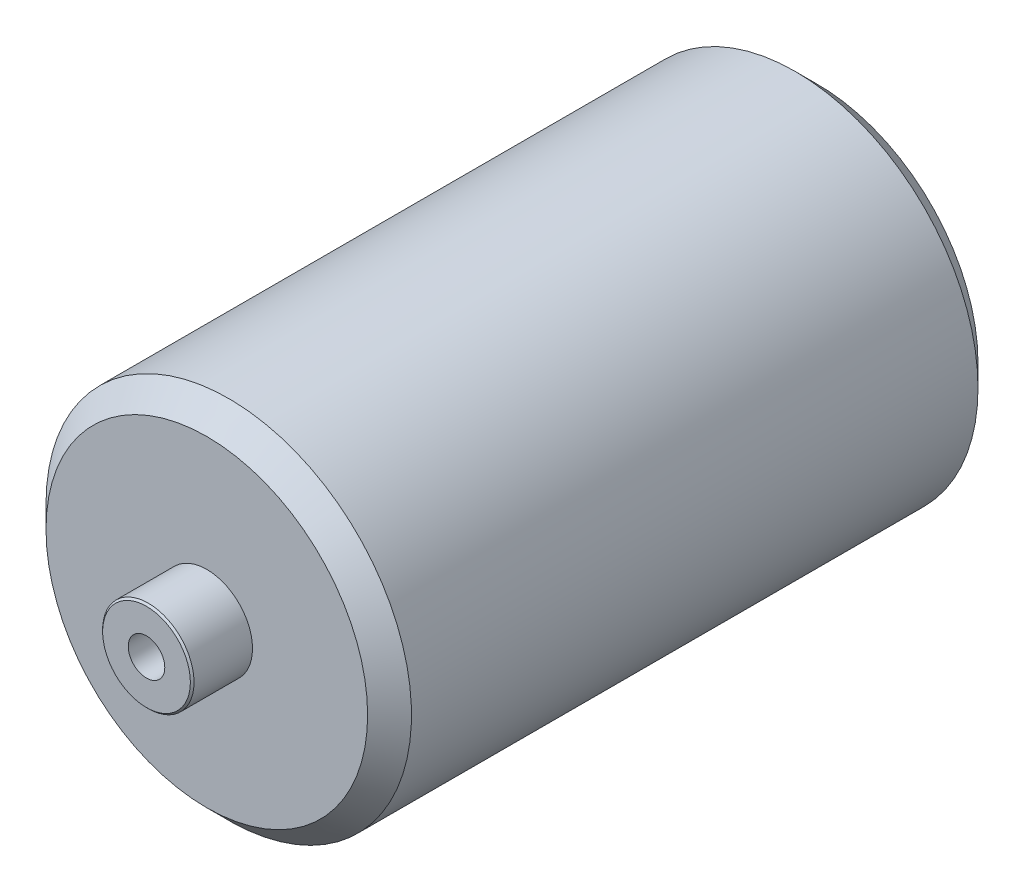
SolidWorks part; units mm, degrees
material "Plain Carbon Steel"
ref_plane "Front Plane" through (0, 0, 0) normal (0, 0, 1) x (1, 0, 0)
ref_plane "Top Plane" through (0, 0, 0) normal (0, 1, 0) x (1, 0, 0)
ref_plane "Right Plane" through (0, 0, 0) normal (1, 0, 0) x (0, 0, -1)
sketch "Body Profile Ø100" plane through (0, 0, 0) normal (0, 0, 1) x (1, 0, 0)
  circle A0 centre (0, 0) radius 50
  dimension "D1" = 100
extrude "Main Body Ø100x167" add sketch "Body Profile Ø100" along normal blind 167
sketch "Spigot 1 Profile Ø25" plane through (0, 0, 167) normal (0, 0, 1) x (1, 0, 0)
  circle A0 centre (0, 0) radius 12.5
  dimension "D1" = 25
extrude "End Spigot 1 Ø25x16.5" add sketch "Spigot 1 Profile Ø25" along normal blind 16.5
sketch "Spigot 2 Profile Ø25" plane through (0, 0, 0) normal (0, 0, -1) x (-1, 0, 0)
  circle A0 centre (0, 0) radius 12.5
  dimension "D1" = 25
extrude "End Spigot 2 Ø25x16.5" add sketch "Spigot 2 Profile Ø25" along normal blind 16.5
sketch "Spigot 2 Dowel Hole Position" plane through (0, 0, -16.5) normal (0, 0, -1) x (-1, 0, 0)
  point P0 (0, 0)
hole_wizard "Spigot 2 Dowel Hole Ø10x59" positions "3DSketch1" profile "Sketch5" hole size "Ø10.0" standard "ISO"
sketch3d "3DSketch1"
  point P0 (0, 0, -16.5)
sketch "Sketch5" plane through (0, 0, -16.5) normal (1, 0, 0) x (0, 1, 0)
  line L0 (0, 0) -> (0, 62.0043)
  line L1 (0, 62.0043) -> (5, 59)
  line L2 (5, 59) -> (5, 0)
  line L5 (5, 0) -> (0, 0)
  line L10 (0, 62.0043) -> (-5, 59) construction
  line L11 (0, -6.35) -> (0, 107.95) construction
  dimension "Hole Dia." = 10
  dimension "Hole Depth" = 59
  dimension "Drill Angle" = 118
sketch "Spigot 1 Dowel Hole Position" plane through (0, 0, 183.5) normal (0, 0, 1) x (1, 0, 0)
  point P0 (0, 0)
hole_wizard "Spigot 1 Dowel Hole Ø10x59" positions "3DSketch3" profile "Sketch9" hole size "Ø10.0" standard "ISO"
sketch3d "3DSketch3"
  point P0 (0, 0, 183.5)
sketch "Sketch9" plane through (0, 0, 183.5) normal (1, 0, 0) x (0, -1, 0)
  line L0 (0, 0) -> (0, 62.0043)
  line L1 (0, 62.0043) -> (5, 59)
  line L2 (5, 59) -> (5, 0)
  line L5 (5, 0) -> (0, 0)
  line L10 (0, 62.0043) -> (-5, 59) construction
  line L11 (0, -6.35) -> (0, 107.95) construction
  dimension "Hole Dia." = 10
  dimension "Hole Depth" = 59
  dimension "Drill Angle" = 118
chamfer "Spigot Edge Chamfer 0.5" distance 0.5 angle 45 2 edges at (-12.5, 0, -16.5) (12.5, 0, 183.5)
chamfer "Body Edge Chamfer 6" distance 6 angle 45 2 edges at (50, 0, 167) (50, 0, 0)
